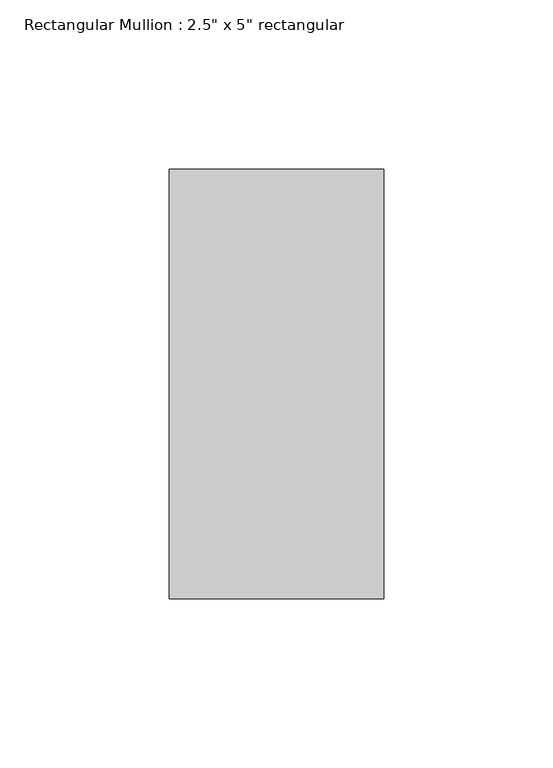
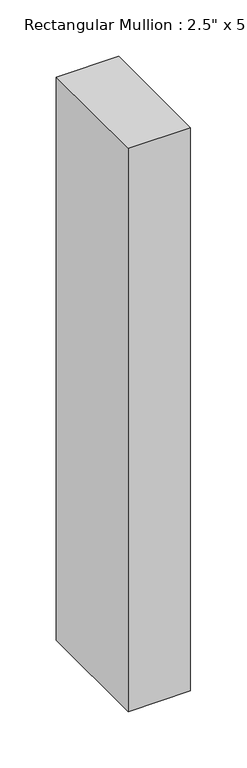
"""IFC4 building model written with IfcOpenShell, lengths in millimetres: member geometry."""

from ifc_helpers import new_model, si_unit, frame, origin, place, context, project, spatial, polyline, outline, extrude, source, transform, mapped, element, save


def member_4a8a2fe5(model_context):
    return source(origin(), model_context, "Body", "SweptSolid", [
        extrude(outline(polyline([(31.75, 63.5), (31.75, -63.5), (-31.75, -63.5), (-31.75, 63.5), (31.75, 63.5)])), frame((0.0, 0.0, -609.1538352), z_axis=(0.0, 0.0, 1.0), x_axis=(1.0, 0.0, 0.0)), (0.0, 0.0, 1.0), 609.1538352),
    ])


if __name__ == "__main__":
    model = new_model("IFC4")
    model_context = context("Model", 3, world=origin())
    ifc_project = project(units=[si_unit("LENGTHUNIT", "METRE", prefix="MILLI")], contexts=[model_context])
    site = spatial("IfcSite", under=ifc_project)
    building = spatial("IfcBuilding", under=site)
    placement = place(None, origin())
    member_shape = member_4a8a2fe5(model_context)
    element("IfcMember", 1, ObjectType="Rectangular Mullion : 2.5\" x 5\" rectangular", at=placement, inside=building, context=model_context, shape_type="MappedRepresentation", body=[
        mapped(member_shape, transform((0.0, 0.0, 0.0), x_axis=(1.0, 0.0, 0.0), y_axis=(0.0, 1.0, 0.0), z_axis=(0.0, 0.0, 1.0))),
    ])
    save(model, "model.ifc")

# Revit data of these elements
# Type "Rectangular Mullion : 2.5\" x 5\" rectangular"
#   built-in parameter 1007304 = 0.416667 (stored number, unit not read)
#   built-in parameter 1007301 = 0.104167 (stored number, unit not read)
#   built-in parameter 1007300 = 0.104167 (stored number, unit not read)
# Element 1 (IfcMember, "Rectangular Mullion : 2.5\" x 5\" rectangular")
#   Materials on its faces: "Aluminum"
# Materials
#   "Aluminum": class "Metal", colour RGB 247 247 247, transparency 0, Description = "Aluminum 6061", Cost = 0
